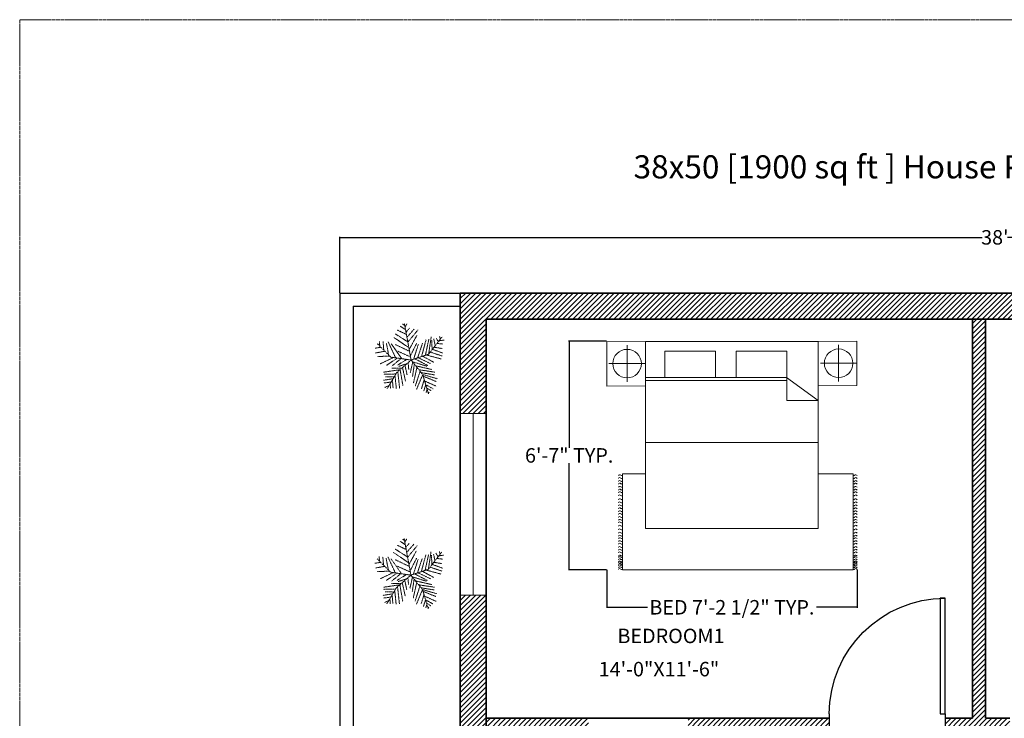
# Model space of a CAD drawing. Units: inches. Extents: x 2202345 to 2203065, y -970921 to -970107.
# Tile 4 of 5: x 2202345 to 2202685, y -970348 to -970107. Entities that reach past the tile are written whole.
import ezdxf

# ---------------------------------------------------------------- set-up
doc = ezdxf.new("R2010")
doc.units = ezdxf.units.IN
doc.header["$MEASUREMENT"] = 0
doc.linetypes.add('HIDDEN', pattern=[0.375, 0.25, -0.125])
doc.layers.get('0').update_dxf_attribs({"color": 13})
for name, color, linetype, lineweight in [('A-ANNO-DIMS', 2, 'Continuous', 18), ('A-ANNO-TEXT', 7, 'Continuous', 25), ('A-ANNO-TTLB', 7, 'HIDDEN', 18), ('A-AREA-IDEN', 7, 'Continuous', 18), ('A-WALL-PATT', 8, 'Continuous', 13), ('C-PROP', 7, 'Continuous', 25), ('doors', 252, 'Continuous', 25), ('furniture', 250, 'Continuous', 18), ('garden', 114, 'HIDDEN', 13), ('walls', 252, 'Continuous', 35), ('windows', 173, 'Continuous', 18)]:
    doc.layers.add(name, color=color, linetype=linetype, lineweight=lineweight)
doc.styles.get("Standard").update_dxf_attribs({"font": 'arial.ttf'})
doc.dimstyles.get("Standard").update_dxf_attribs({"dimtxt": 5, "dimasz": 0.18, "dimexe": 0.18, "dimexo": 0.0625, "dimgap": 0.09, "dimtad": 0, "dimtih": 1, "dimtoh": 1, "dimzin": 0, "dimdsep": 46, "dimlunit": 3, "dimtxsty": 'Standard', "dimcen": 0.09, "dimadec": 0, "dimazin": 0, "dimtfac": 1, "dimtofl": 0, "dimtmove": 0, "dimatfit": 3, "dimfxl": 1, "dimtolj": 1, "dimtzin": 0, "dimarcsym": 0})

# ---------------------------------------------------------------- blocks, each defined once
blk = doc.blocks.new('CARPET')
at = {"layer": 'furniture'}
for p, q in [((-51.53, -98.11), (-51.53, -55.12)), ((-51.53, -55.12), (-41.27, -55.12)), ((36, -55.12), (51.55, -55.12)), ((51.55, -55.12), (51.55, -98.11)), ((51.55, -98.11), (-51.53, -98.11))]:
    blk.add_line(p, q, dxfattribs=at)
for points, knots in [([(-53.37, -55.99), (-53.22, -55.8), (-52.9, -55.41), (-52.34, -55.8), (-51.89, -56.08), (-51.65, -55.91), (-51.53, -55.83)], [0, 0, 0, 0, 0.653278, 1.290138, 1.740457, 2.114451, 2.114451, 2.114451, 2.114451]), ([(-53.37, -57.26), (-53.22, -57.07), (-52.9, -56.67), (-52.34, -57.07), (-51.89, -57.35), (-51.65, -57.17), (-51.53, -57.1)], [0, 0, 0, 0, 0.653278, 1.290138, 1.740457, 2.114451, 2.114451, 2.114451, 2.114451]), ([(53.37, -55.99), (53.22, -55.8), (52.9, -55.41), (52.34, -55.8), (51.89, -56.08), (51.65, -55.91), (51.53, -55.83)], [0, 0, 0, 0, 0.653278, 1.290138, 1.740457, 2.114451, 2.114451, 2.114451, 2.114451]), ([(53.37, -57.26), (53.22, -57.07), (52.9, -56.67), (52.34, -57.07), (51.89, -57.35), (51.65, -57.17), (51.53, -57.1)], [0, 0, 0, 0, 0.653278, 1.290138, 1.740457, 2.114451, 2.114451, 2.114451, 2.114451]), ([(-53.37, -58.59), (-53.22, -58.4), (-52.9, -58.01), (-52.34, -58.4), (-51.89, -58.68), (-51.65, -58.5), (-51.53, -58.43)], [0, 0, 0, 0, 0.653278, 1.290138, 1.740457, 2.114451, 2.114451, 2.114451, 2.114451]), ([(-53.37, -59.78), (-53.22, -59.58), (-52.9, -59.19), (-52.34, -59.58), (-51.89, -59.86), (-51.65, -59.69), (-51.53, -59.61)], [0, 0, 0, 0, 0.653278, 1.290138, 1.740457, 2.114451, 2.114451, 2.114451, 2.114451]), ([(-53.37, -61.22), (-53.22, -61.02), (-52.9, -60.63), (-52.34, -61.02), (-51.89, -61.3), (-51.65, -61.13), (-51.53, -61.05)], [0, 0, 0, 0, 0.653278, 1.290138, 1.740457, 2.114451, 2.114451, 2.114451, 2.114451]), ([(53.37, -58.59), (53.22, -58.4), (52.9, -58.01), (52.34, -58.4), (51.89, -58.68), (51.65, -58.5), (51.53, -58.43)], [0, 0, 0, 0, 0.653278, 1.290138, 1.740457, 2.114451, 2.114451, 2.114451, 2.114451]), ([(53.37, -59.78), (53.22, -59.58), (52.9, -59.19), (52.34, -59.58), (51.89, -59.86), (51.65, -59.69), (51.53, -59.61)], [0, 0, 0, 0, 0.653278, 1.290138, 1.740457, 2.114451, 2.114451, 2.114451, 2.114451]), ([(53.37, -61.22), (53.22, -61.02), (52.9, -60.63), (52.34, -61.02), (51.89, -61.3), (51.65, -61.13), (51.53, -61.05)], [0, 0, 0, 0, 0.653278, 1.290138, 1.740457, 2.114451, 2.114451, 2.114451, 2.114451]), ([(-53.37, -62.44), (-53.22, -62.25), (-52.9, -61.86), (-52.34, -62.25), (-51.89, -62.53), (-51.65, -62.36), (-51.53, -62.28)], [0, 0, 0, 0, 0.653278, 1.290138, 1.740457, 2.114451, 2.114451, 2.114451, 2.114451]), ([(-53.37, -63.63), (-53.22, -63.43), (-52.9, -63.04), (-52.34, -63.43), (-51.89, -63.72), (-51.65, -63.54), (-51.53, -63.46)], [0, 0, 0, 0, 0.653278, 1.290138, 1.740457, 2.114451, 2.114451, 2.114451, 2.114451]), ([(-53.37, -65.07), (-53.22, -64.87), (-52.9, -64.48), (-52.34, -64.87), (-51.89, -65.15), (-51.65, -64.98), (-51.53, -64.9)], [0, 0, 0, 0, 0.653278, 1.290138, 1.740457, 2.114451, 2.114451, 2.114451, 2.114451]), ([(53.37, -62.44), (53.22, -62.25), (52.9, -61.86), (52.34, -62.25), (51.89, -62.53), (51.65, -62.36), (51.53, -62.28)], [0, 0, 0, 0, 0.653278, 1.290138, 1.740457, 2.114451, 2.114451, 2.114451, 2.114451]), ([(53.37, -63.63), (53.22, -63.43), (52.9, -63.04), (52.34, -63.43), (51.89, -63.72), (51.65, -63.54), (51.53, -63.46)], [0, 0, 0, 0, 0.653278, 1.290138, 1.740457, 2.114451, 2.114451, 2.114451, 2.114451]), ([(53.37, -65.07), (53.22, -64.87), (52.9, -64.48), (52.34, -64.87), (51.89, -65.15), (51.65, -64.98), (51.53, -64.9)], [0, 0, 0, 0, 0.653278, 1.290138, 1.740457, 2.114451, 2.114451, 2.114451, 2.114451]), ([(-53.37, -66.76), (-53.22, -66.56), (-52.9, -66.17), (-52.34, -66.56), (-51.89, -66.84), (-51.65, -66.67), (-51.53, -66.59)], [0, 0, 0, 0, 0.653278, 1.290138, 1.740457, 2.114451, 2.114451, 2.114451, 2.114451]), ([(-53.37, -68.2), (-53.22, -68), (-52.9, -67.61), (-52.34, -68), (-51.89, -68.28), (-51.65, -68.11), (-51.53, -68.03)], [0, 0, 0, 0, 0.653278, 1.290138, 1.740457, 2.114451, 2.114451, 2.114451, 2.114451]), ([(-53.37, -69.53), (-53.22, -69.33), (-52.9, -68.94), (-52.34, -69.33), (-51.89, -69.61), (-51.65, -69.44), (-51.53, -69.36)], [0, 0, 0, 0, 0.653278, 1.290138, 1.740457, 2.114451, 2.114451, 2.114451, 2.114451]), ([(-53.37, -70.79), (-53.22, -70.6), (-52.9, -70.21), (-52.34, -70.6), (-51.89, -70.88), (-51.65, -70.7), (-51.53, -70.63)], [0, 0, 0, 0, 0.653278, 1.290138, 1.740457, 2.114451, 2.114451, 2.114451, 2.114451]), ([(53.37, -66.76), (53.22, -66.56), (52.9, -66.17), (52.34, -66.56), (51.89, -66.84), (51.65, -66.67), (51.53, -66.59)], [0, 0, 0, 0, 0.653278, 1.290138, 1.740457, 2.114451, 2.114451, 2.114451, 2.114451]), ([(53.37, -68.2), (53.22, -68), (52.9, -67.61), (52.34, -68), (51.89, -68.28), (51.65, -68.11), (51.53, -68.03)], [0, 0, 0, 0, 0.653278, 1.290138, 1.740457, 2.114451, 2.114451, 2.114451, 2.114451]), ([(53.37, -69.53), (53.22, -69.33), (52.9, -68.94), (52.34, -69.33), (51.89, -69.61), (51.65, -69.44), (51.53, -69.36)], [0, 0, 0, 0, 0.653278, 1.290138, 1.740457, 2.114451, 2.114451, 2.114451, 2.114451]), ([(53.37, -70.79), (53.22, -70.6), (52.9, -70.21), (52.34, -70.6), (51.89, -70.88), (51.65, -70.7), (51.53, -70.63)], [0, 0, 0, 0, 0.653278, 1.290138, 1.740457, 2.114451, 2.114451, 2.114451, 2.114451]), ([(-53.37, -72.12), (-53.22, -71.93), (-52.9, -71.54), (-52.34, -71.93), (-51.89, -72.21), (-51.65, -72.04), (-51.53, -71.96)], [0, 0, 0, 0, 0.653278, 1.290138, 1.740457, 2.114451, 2.114451, 2.114451, 2.114451]), ([(-53.37, -73.31), (-53.22, -73.11), (-52.9, -72.72), (-52.34, -73.11), (-51.89, -73.4), (-51.65, -73.22), (-51.53, -73.14)], [0, 0, 0, 0, 0.653278, 1.290138, 1.740457, 2.114451, 2.114451, 2.114451, 2.114451]), ([(-53.37, -74.75), (-53.22, -74.55), (-52.9, -74.16), (-52.34, -74.55), (-51.89, -74.83), (-51.65, -74.66), (-51.53, -74.58)], [0, 0, 0, 0, 0.653278, 1.290138, 1.740457, 2.114451, 2.114451, 2.114451, 2.114451]), ([(53.37, -72.12), (53.22, -71.93), (52.9, -71.54), (52.34, -71.93), (51.89, -72.21), (51.65, -72.04), (51.53, -71.96)], [0, 0, 0, 0, 0.653278, 1.290138, 1.740457, 2.114451, 2.114451, 2.114451, 2.114451]), ([(53.37, -73.31), (53.22, -73.11), (52.9, -72.72), (52.34, -73.11), (51.89, -73.4), (51.65, -73.22), (51.53, -73.14)], [0, 0, 0, 0, 0.653278, 1.290138, 1.740457, 2.114451, 2.114451, 2.114451, 2.114451]), ([(53.37, -74.75), (53.22, -74.55), (52.9, -74.16), (52.34, -74.55), (51.89, -74.83), (51.65, -74.66), (51.53, -74.58)], [0, 0, 0, 0, 0.653278, 1.290138, 1.740457, 2.114451, 2.114451, 2.114451, 2.114451]), ([(-53.37, -75.98), (-53.22, -75.78), (-52.9, -75.39), (-52.34, -75.78), (-51.89, -76.06), (-51.65, -75.89), (-51.53, -75.81)], [0, 0, 0, 0, 0.653278, 1.290138, 1.740457, 2.114451, 2.114451, 2.114451, 2.114451]), ([(-53.37, -77.16), (-53.22, -76.96), (-52.9, -76.57), (-52.34, -76.96), (-51.89, -77.25), (-51.65, -77.07), (-51.53, -76.99)], [0, 0, 0, 0, 0.653278, 1.290138, 1.740457, 2.114451, 2.114451, 2.114451, 2.114451]), ([(-53.37, -78.6), (-53.22, -78.4), (-52.9, -78.01), (-52.34, -78.4), (-51.89, -78.68), (-51.65, -78.51), (-51.53, -78.43)], [0, 0, 0, 0, 0.653278, 1.290138, 1.740457, 2.114451, 2.114451, 2.114451, 2.114451]), ([(53.37, -75.98), (53.22, -75.78), (52.9, -75.39), (52.34, -75.78), (51.89, -76.06), (51.65, -75.89), (51.53, -75.81)], [0, 0, 0, 0, 0.653278, 1.290138, 1.740457, 2.114451, 2.114451, 2.114451, 2.114451]), ([(53.37, -77.16), (53.22, -76.96), (52.9, -76.57), (52.34, -76.96), (51.89, -77.25), (51.65, -77.07), (51.53, -76.99)], [0, 0, 0, 0, 0.653278, 1.290138, 1.740457, 2.114451, 2.114451, 2.114451, 2.114451]), ([(53.37, -78.6), (53.22, -78.4), (52.9, -78.01), (52.34, -78.4), (51.89, -78.68), (51.65, -78.51), (51.53, -78.43)], [0, 0, 0, 0, 0.653278, 1.290138, 1.740457, 2.114451, 2.114451, 2.114451, 2.114451]), ([(-53.37, -80.29), (-53.22, -80.09), (-52.9, -79.7), (-52.34, -80.09), (-51.89, -80.37), (-51.65, -80.2), (-51.53, -80.12)], [0, 0, 0, 0, 0.653278, 1.290138, 1.740457, 2.114451, 2.114451, 2.114451, 2.114451]), ([(-53.37, -81.73), (-53.22, -81.53), (-52.9, -81.14), (-52.34, -81.53), (-51.89, -81.81), (-51.65, -81.64), (-51.53, -81.56)], [0, 0, 0, 0, 0.653278, 1.290138, 1.740457, 2.114451, 2.114451, 2.114451, 2.114451]), ([(-53.37, -83.06), (-53.22, -82.86), (-52.9, -82.47), (-52.34, -82.86), (-51.89, -83.14), (-51.65, -82.97), (-51.53, -82.89)], [0, 0, 0, 0, 0.653278, 1.290138, 1.740457, 2.114451, 2.114451, 2.114451, 2.114451]), ([(53.37, -80.29), (53.22, -80.09), (52.9, -79.7), (52.34, -80.09), (51.89, -80.37), (51.65, -80.2), (51.53, -80.12)], [0, 0, 0, 0, 0.653278, 1.290138, 1.740457, 2.114451, 2.114451, 2.114451, 2.114451]), ([(53.37, -81.73), (53.22, -81.53), (52.9, -81.14), (52.34, -81.53), (51.89, -81.81), (51.65, -81.64), (51.53, -81.56)], [0, 0, 0, 0, 0.653278, 1.290138, 1.740457, 2.114451, 2.114451, 2.114451, 2.114451]), ([(53.37, -83.06), (53.22, -82.86), (52.9, -82.47), (52.34, -82.86), (51.89, -83.14), (51.65, -82.97), (51.53, -82.89)], [0, 0, 0, 0, 0.653278, 1.290138, 1.740457, 2.114451, 2.114451, 2.114451, 2.114451]), ([(-53.37, -84.18), (-53.22, -83.99), (-52.9, -83.6), (-52.34, -83.99), (-51.89, -84.27), (-51.65, -84.09), (-51.53, -84.02)], [0, 0, 0, 0, 0.653278, 1.290138, 1.740457, 2.114451, 2.114451, 2.114451, 2.114451]), ([(-53.37, -85.51), (-53.22, -85.32), (-52.9, -84.93), (-52.34, -85.32), (-51.89, -85.6), (-51.65, -85.42), (-51.53, -85.35)], [0, 0, 0, 0, 0.653278, 1.290138, 1.740457, 2.114451, 2.114451, 2.114451, 2.114451]), ([(-53.37, -86.7), (-53.22, -86.5), (-52.9, -86.11), (-52.34, -86.5), (-51.89, -86.78), (-51.65, -86.61), (-51.53, -86.53)], [0, 0, 0, 0, 0.653278, 1.290138, 1.740457, 2.114451, 2.114451, 2.114451, 2.114451]), ([(-53.37, -88.14), (-53.22, -87.94), (-52.9, -87.55), (-52.34, -87.94), (-51.89, -88.22), (-51.65, -88.05), (-51.53, -87.97)], [0, 0, 0, 0, 0.653278, 1.290138, 1.740457, 2.114451, 2.114451, 2.114451, 2.114451]), ([(53.37, -84.18), (53.22, -83.99), (52.9, -83.6), (52.34, -83.99), (51.89, -84.27), (51.65, -84.09), (51.53, -84.02)], [0, 0, 0, 0, 0.653278, 1.290138, 1.740457, 2.114451, 2.114451, 2.114451, 2.114451]), ([(53.37, -85.51), (53.22, -85.32), (52.9, -84.93), (52.34, -85.32), (51.89, -85.6), (51.65, -85.42), (51.53, -85.35)], [0, 0, 0, 0, 0.653278, 1.290138, 1.740457, 2.114451, 2.114451, 2.114451, 2.114451]), ([(53.37, -86.7), (53.22, -86.5), (52.9, -86.11), (52.34, -86.5), (51.89, -86.78), (51.65, -86.61), (51.53, -86.53)], [0, 0, 0, 0, 0.653278, 1.290138, 1.740457, 2.114451, 2.114451, 2.114451, 2.114451]), ([(53.37, -88.14), (53.22, -87.94), (52.9, -87.55), (52.34, -87.94), (51.89, -88.22), (51.65, -88.05), (51.53, -87.97)], [0, 0, 0, 0, 0.653278, 1.290138, 1.740457, 2.114451, 2.114451, 2.114451, 2.114451]), ([(-53.37, -89.36), (-53.22, -89.17), (-52.9, -88.78), (-52.34, -89.17), (-51.89, -89.45), (-51.65, -89.28), (-51.53, -89.2)], [0, 0, 0, 0, 0.653278, 1.290138, 1.740457, 2.114451, 2.114451, 2.114451, 2.114451]), ([(-53.37, -90.55), (-53.22, -90.35), (-52.9, -89.96), (-52.34, -90.35), (-51.89, -90.64), (-51.65, -90.46), (-51.53, -90.38)], [0, 0, 0, 0, 0.653278, 1.290138, 1.740457, 2.114451, 2.114451, 2.114451, 2.114451]), ([(-53.37, -91.99), (-53.22, -91.79), (-52.9, -91.4), (-52.34, -91.79), (-51.89, -92.07), (-51.65, -91.9), (-51.53, -91.82)], [0, 0, 0, 0, 0.653278, 1.290138, 1.740457, 2.114451, 2.114451, 2.114451, 2.114451]), ([(-53.37, -92.69), (-53.22, -92.48), (-52.9, -92.08), (-52.35, -92.49), (-51.89, -92.77), (-51.65, -92.6), (-51.53, -92.52)], [0, 0, 0, 0, 0.663904, 1.307406, 1.757725, 2.131719, 2.131719, 2.131719, 2.131719]), ([(53.37, -89.36), (53.22, -89.17), (52.9, -88.78), (52.34, -89.17), (51.89, -89.45), (51.65, -89.28), (51.53, -89.2)], [0, 0, 0, 0, 0.653278, 1.290138, 1.740457, 2.114451, 2.114451, 2.114451, 2.114451]), ([(53.37, -90.55), (53.22, -90.35), (52.9, -89.96), (52.34, -90.35), (51.9, -90.63), (51.66, -90.47), (51.55, -90.4)], [0, 0, 0, 0, 0.653278, 1.290138, 1.740457, 2.0926, 2.0926, 2.0926, 2.0926]), ([(53.37, -91.99), (53.22, -91.79), (52.9, -91.4), (52.34, -91.79), (51.9, -92.07), (51.66, -91.91), (51.55, -91.83)], [0, 0, 0, 0, 0.653278, 1.290138, 1.740457, 2.0926, 2.0926, 2.0926, 2.0926]), ([(53.37, -92.69), (53.22, -92.49), (52.9, -92.09), (52.34, -92.49), (51.9, -92.77), (51.66, -92.61), (51.55, -92.53)], [0, 0, 0, 0, 0.656792, 1.295826, 1.746145, 2.098292, 2.098292, 2.098292, 2.098292]), ([(-53.37, -93.61), (-53.22, -93.42), (-52.9, -93.03), (-52.34, -93.42), (-51.89, -93.7), (-51.65, -93.52), (-51.53, -93.45)], [0, 0, 0, 0, 0.653278, 1.290138, 1.740457, 2.114451, 2.114451, 2.114451, 2.114451]), ([(-53.37, -94.55), (-53.22, -94.35), (-52.9, -93.96), (-52.34, -94.35), (-51.89, -94.63), (-51.65, -94.46), (-51.53, -94.38)], [0, 0, 0, 0, 0.653278, 1.290138, 1.740457, 2.114451, 2.114451, 2.114451, 2.114451]), ([(-53.37, -95.05), (-53.22, -94.85), (-52.9, -94.46), (-52.34, -94.85), (-51.89, -95.14), (-51.65, -94.96), (-51.53, -94.88)], [0, 0, 0, 0, 0.653278, 1.290138, 1.740457, 2.114451, 2.114451, 2.114451, 2.114451]), ([(-53.37, -95.73), (-53.22, -95.54), (-52.9, -95.15), (-52.34, -95.54), (-51.89, -95.82), (-51.65, -95.65), (-51.53, -95.57)], [0, 0, 0, 0, 0.653278, 1.290138, 1.740457, 2.114451, 2.114451, 2.114451, 2.114451]), ([(-53.37, -96.38), (-53.22, -96.18), (-52.9, -95.79), (-52.34, -96.18), (-51.89, -96.47), (-51.65, -96.29), (-51.53, -96.21)], [0, 0, 0, 0, 0.653278, 1.290138, 1.740457, 2.114451, 2.114451, 2.114451, 2.114451]), ([(-53.37, -97.17), (-53.22, -96.98), (-52.9, -96.59), (-52.34, -96.98), (-51.89, -97.26), (-51.65, -97.08), (-51.53, -97.01)], [0, 0, 0, 0, 0.653278, 1.290138, 1.740457, 2.114451, 2.114451, 2.114451, 2.114451]), ([(53.37, -95.78), (53.22, -95.58), (52.9, -95.19), (52.34, -95.58), (51.89, -95.86), (51.65, -95.69), (51.53, -95.61)], [0, 0, 0, 0, 0.653278, 1.290138, 1.740457, 2.114451, 2.114451, 2.114451, 2.114451]), ([(53.37, -96.43), (53.22, -96.23), (52.9, -95.84), (52.34, -96.23), (51.89, -96.51), (51.65, -96.34), (51.53, -96.26)], [0, 0, 0, 0, 0.653278, 1.290138, 1.740457, 2.114451, 2.114451, 2.114451, 2.114451]), ([(53.37, -97.22), (53.22, -97.02), (52.9, -96.63), (52.34, -97.02), (51.89, -97.3), (51.65, -97.13), (51.53, -97.05)], [0, 0, 0, 0, 0.653278, 1.290138, 1.740457, 2.114451, 2.114451, 2.114451, 2.114451]), ([(53.37, -93.66), (53.22, -93.46), (52.9, -93.07), (52.34, -93.46), (51.9, -93.74), (51.66, -93.58), (51.55, -93.5)], [0, 0, 0, 0, 0.653278, 1.290138, 1.740457, 2.0926, 2.0926, 2.0926, 2.0926]), ([(53.37, -94.59), (53.22, -94.4), (52.9, -94.01), (52.34, -94.4), (51.9, -94.68), (51.66, -94.51), (51.55, -94.44)], [0, 0, 0, 0, 0.653278, 1.290138, 1.740457, 2.0926, 2.0926, 2.0926, 2.0926]), ([(53.37, -95.1), (53.22, -94.9), (52.9, -94.51), (52.34, -94.9), (51.9, -95.18), (51.66, -95.02), (51.55, -94.94)], [0, 0, 0, 0, 0.653278, 1.290138, 1.740457, 2.0926, 2.0926, 2.0926, 2.0926]), ([(-53.37, -97.99), (-53.22, -97.79), (-52.9, -97.4), (-52.34, -97.79), (-51.89, -98.08), (-51.65, -97.9), (-51.53, -97.82)], [0, 0, 0, 0, 0.653278, 1.290138, 1.740457, 2.114451, 2.114451, 2.114451, 2.114451]), ([(53.37, -97.99), (53.22, -97.79), (52.9, -97.4), (52.34, -97.79), (51.89, -98.08), (51.65, -97.9), (51.53, -97.82)], [0, 0, 0, 0, 0.653278, 1.290138, 1.740457, 2.114451, 2.114451, 2.114451, 2.114451])]:
    blk.add_open_spline(points, degree=3, knots=knots, dxfattribs=at)
blk = doc.blocks.new('A$C58D270C6')
at = {"layer": 'furniture'}
for p, q in [((9.09, 124.13), (9.09, 108.87)), ((1.46, 116.5), (16.73, 116.5)), ((14.97, 94.84), (24.62, 107.92)), ((24.62, 94.93), (24.62, 107.92)), ((42.08, 108), (42.08, 36)), ((14.97, 94.93), (24.62, 94.93)), ((14.97, 94.84), (14.97, 36)), ((16.22, 94.93), (16.22, 36)), ((9.25, 36), (9.25, 20.74)), ((1.62, 28.37), (16.88, 28.37))]:
    blk.add_line(p, q, dxfattribs=at)
for points in [[(18.5, 108), (18.34, 124.13), (-0.16, 124.13), (0, 108)], [(0, 108), (77.91, 108), (77.91, 36), (0, 36)], [(4.09, 94.93), (14.97, 94.93), (14.97, 73.83), (4.09, 73.83)], [(4.09, 65.23), (14.97, 65.23), (14.97, 44.13), (4.09, 44.13)], [(18.65, 19.87), (18.5, 36), (0, 36), (0.16, 19.87)]]:
    blk.add_lwpolyline(points, close=True, dxfattribs=at)
for centre in [(9.09, 116.5), (9.25, 28.37)]:
    blk.add_circle(centre, 5.95, dxfattribs=at)
at = {"layer": 'furniture', "xscale": 0.9312884925094044, "yscale": 0.9312884925094044, "zscale": 0.9312884925094044, "rotation": 90}
blk.add_blockref('CARPET', (3.79, 74.47), dxfattribs=at)
blk = doc.blocks.new('*U12')
for p, q in [((0, 0), (0, -6)), ((40, 0), (40, -6))]:
    blk.add_line(p, q)
blk.add_lwpolyline([(0, 0), (0, 40), (1.75, 40), (1.75, 0)], close=True)
blk.add_arc((0, 0), 40, 0, 90)
blk = doc.blocks.new('*D20')
at = {"layer": 'A-ANNO-DIMS', "color": 0, "lineweight": -2, "transparency": 16777216}
for p, q in [((2202455.18, -970201.04), (2202455.18, -970181.68)), ((2202455.36, -970181.86), (2202677.1, -970181.86)), ((2202907.5, -970181.86), (2202685.76, -970181.86)), ((2202907.68, -970201.04), (2202907.68, -970181.68))]:
    blk.add_line(p, q, dxfattribs=at)
at = {"layer": 'A-ANNO-DIMS', "color": 0, "transparency": 16777216}
for points in [[(2202455.36, -970181.83), (2202455.36, -970181.89), (2202455.18, -970181.86)], [(2202907.5, -970181.83), (2202907.5, -970181.89), (2202907.68, -970181.86)]]:
    blk.add_solid(points, dxfattribs=at)
at = {"layer": 'Defpoints', "color": 0, "transparency": 16777216}
for p in [(2202907.68, -970181.86), (2202455.18, -970201.11), (2202907.68, -970201.11)]:
    blk.add_point(p, dxfattribs=at)
at = {"layer": 'A-ANNO-DIMS', "color": 0, "transparency": 16777216, "insert": (2202681.43, -970181.86), "char_height": 5, "attachment_point": 5}
blk.add_mtext("\\A1;38'", dxfattribs=at)
blk = doc.blocks.new('*U23')
for p, q in [((-7.288, 39.707), (-21.778, 46.673)), ((-8.737, 47.138), (-17.069, 52.711)), ((-10.186, 53.64), (-13.084, 55.962)), ((0, 0), (-10.5, 57)), ((-9.099, 51.782), (-6.563, 55.962)), ((-7.65, 43.423), (-2.578, 49.46)), ((-5.839, 35.992), (4.667, 48.067)), ((-5.114, 27.632), (10.463, 46.673)), ((-3.665, 19.273), (-27.574, 35.527)), ((-5.114, 28.097), (-24.676, 40.636)), ((-2.941, 16.486), (8.652, 37.85)), ((16.259, 5.805), (23.142, 31.348)), ((22.055, 7.198), (27.489, 32.277)), ((27, 9), (48, 36)), ((27.127, 9.056), (31.112, 35.992)), ((31.836, 30.883), (32.561, 16.486)), ((35.096, 32.741), (37.27, 22.524)), ((38.719, 34.134), (41.979, 28.561)), ((43.791, 29.954), (51.036, 30.883)), ((44.153, 36.456), (45.239, 32.741)), ((-47.498, 19.737), (-55.83, 18.344)), ((-31.5, 4.5), (-52.5, 25.5)), ((-48.585, 21.131), (-49.309, 29.026)), ((-43.513, 28.561), (-42.427, 15.558)), ((-38.442, 26.239), (-34.819, 7.663)), ((-35.544, 28.097), (-24.314, 3.947)), ((-14.533, 2.09), (-30.834, 25.31)), ((-24.314, 23.917), (-2.941, 13.7)), ((-1.129, 6.734), (9.014, 26.704)), ((3.942, 1.625), (11.187, 24.381)), ((10.101, 3.483), (17.708, 26.239)), ((33.285, 16.486), (48.862, 10.913)), ((36.183, 19.737), (48.137, 17.88)), ((40.53, 25.775), (48.862, 24.846)), ((-40.615, 13.7), (-55.105, 10.913)), ((-33.37, 6.269), (-52.207, 5.34)), ((-28.299, 3.483), (-47.86, -5.805)), ((-21.416, 3.018), (-38.079, -8.128)), ((0, 0), (-31.5, 4.5)), ((-15.982, 2.09), (-30.11, -9.521)), ((0, 0), (-22.5, -19.5)), ((-6.563, 1.161), (-21.416, -8.128)), ((-20.691, 13.7), (-1.129, 4.876)), ((0, 0), (27, 9)), ((0, 0), (18, -22.5)), ((6.478, 1.625), (26.04, -8.592)), ((11.187, 3.483), (30.749, -5.805)), ((18.07, 5.805), (35.096, -3.483)), ((24.229, 7.663), (46.688, 1.625)), ((29.662, 12.307), (48.137, 6.269)), ((-17.431, -15.094), (-42.789, -18.809)), ((-15.257, -12.772), (-30.11, -12.772)), ((-6.563, -5.805), (-19.967, -9.985)), ((-17.069, -15.094), (-12.721, -40.172)), ((-13.446, -11.378), (-8.737, -32.741)), ((-9.461, -8.592), (-6.201, -23.453)), ((-4.752, -3.483), (-3.665, -14.629)), ((2.493, -3.019), (-1.491, -20.202)), ((1.769, -2.555), (24.229, -9.521)), ((5.029, -6.27), (2.131, -25.775)), ((9.014, -11.378), (3.58, -35.992)), ((7.565, -9.056), (32.198, -14.629)), ((12.274, -15.094), (36.907, -18.809)), ((-28.299, -29.026), (-42.789, -31.348)), ((-24.314, -21.596), (-42.427, -22.06)), ((-26.849, -26.24), (-40.253, -25.775)), ((-22.5, -19.5), (-37.5, -45)), ((-25.038, -23.918), (-22.865, -45.281)), ((-20.691, -18.345), (-17.793, -44.352)), ((14.085, -16.951), (6.478, -40.172)), ((18.07, -22.524), (8.289, -45.745)), ((20.244, -30.419), (15.897, -44.816)), ((16.259, -19.738), (36.183, -22.989)), ((18, -22.5), (27, -52.5)), ((18.433, -22.524), (40.53, -29.026)), ((19.157, -25.311), (38.719, -33.206)), ((-30.834, -34.135), (-42.427, -35.528)), ((-34.457, -39.708), (-40.978, -42.494)), ((-32.646, -36.921), (-31.921, -44.352)), ((-29.023, -30.884), (-27.936, -43.887)), ((22.78, -37.85), (19.519, -48.532)), ((21.331, -32.741), (39.081, -40.636)), ((22.78, -38.314), (34.372, -44.816)), ((24.591, -45.745), (23.142, -50.854)), ((24.591, -43.423), (30.749, -47.603)), ((26.764, -49.925), (28.213, -50.854))]:
    blk.add_line(p, q)
blk = doc.blocks.new('*D25')
at = {"layer": 'A-ANNO-DIMS', "color": 0, "lineweight": -2, "transparency": 16777216}
for p, q in [((2202547.33, -970296.82), (2202547.33, -970309.91)), ((2202633.84, -970296.82), (2202633.84, -970309.91)), ((2202547.51, -970309.73), (2202561.39, -970309.73)), ((2202633.66, -970309.73), (2202619.78, -970309.73))]:
    blk.add_line(p, q, dxfattribs=at)
at = {"layer": 'A-ANNO-DIMS', "color": 0, "transparency": 16777216}
for points in [[(2202547.51, -970309.7), (2202547.51, -970309.76), (2202547.33, -970309.73)], [(2202633.66, -970309.7), (2202633.66, -970309.76), (2202633.84, -970309.73)]]:
    blk.add_solid(points, dxfattribs=at)
at = {"layer": 'Defpoints', "color": 0, "transparency": 16777216}
for p in [(2202547.33, -970296.75), (2202633.84, -970296.75), (2202633.84, -970309.73)]:
    blk.add_point(p, dxfattribs=at)
at = {"layer": 'A-ANNO-DIMS', "color": 0, "transparency": 16777216, "insert": (2202590.58, -970309.73), "char_height": 5, "attachment_point": 5}
blk.add_mtext('\\A1;BED 7\'-2 1/2" TYP.', dxfattribs=at)
blk = doc.blocks.new('*D26')
at = {"layer": 'A-ANNO-DIMS', "color": 0, "lineweight": -2, "transparency": 16777216}
for p, q in [((2202547.27, -970217.71), (2202534.18, -970217.71)), ((2202534.36, -970217.89), (2202534.36, -970254.59)), ((2202534.36, -970296.57), (2202534.36, -970259.88)), ((2202547.27, -970296.75), (2202534.18, -970296.75))]:
    blk.add_line(p, q, dxfattribs=at)
at = {"layer": 'A-ANNO-DIMS', "color": 0, "transparency": 16777216}
for points in [[(2202534.33, -970217.89), (2202534.39, -970217.89), (2202534.36, -970217.71)], [(2202534.33, -970296.57), (2202534.39, -970296.57), (2202534.36, -970296.75)]]:
    blk.add_solid(points, dxfattribs=at)
at = {"layer": 'Defpoints', "color": 0, "transparency": 16777216}
for p in [(2202547.33, -970217.71), (2202534.36, -970296.75), (2202547.33, -970296.75)]:
    blk.add_point(p, dxfattribs=at)
at = {"layer": 'A-ANNO-DIMS', "color": 0, "transparency": 16777216, "insert": (2202534.36, -970257.23), "char_height": 5, "attachment_point": 5}
blk.add_mtext('\\A1;6\'-7" TYP.', dxfattribs=at)

msp = doc.modelspace()

# ---------------------------------------------------------------- hatches: boundary and pattern name
at = {"layer": 'A-WALL-PATT'}
h = msp.add_hatch(dxfattribs=at)
h.set_pattern_fill('ANSI31', color=256, scale=10)
h.set_pattern_definition([(45, (0, 0), (-0.8838834765, 0.8838834765), [])])
h.paths.add_polyline_path([(2202648.182, -970512.768), (2202644.707, -970512.768, -0.0110733), (2202643.682, -970512.746), (2202643.682, -970601.606), (2202609.913, -970601.606), (2202609.913, -970610.606), (2202643.682, -970610.606), (2202643.682, -970619.168), (2202647.677, -970619.168, -0.0047326), (2202648.182, -970619.173)])
h.paths.add_polyline_path([(2202643.682, -970610.606), (2202636.037, -970610.606), (2202636.037, -970659.106), (2202643.682, -970659.106)])
h.paths.add_polyline_path([(2202722.39, -970654.606), (2202722.39, -970650.106), (2202648.182, -970650.106), (2202648.182, -970645.806), (2202647.677, -970645.806), (2202643.682, -970645.806), (2202643.682, -970659.106), (2202722.39, -970659.106)])
h.paths.add_polyline_path([(2202846.182, -970650.106), (2202798.148, -970650.106), (2202798.148, -970659.106), (2202846.182, -970659.106)])
h.paths.add_polyline_path([(2202855.182, -970619.995), (2202846.182, -970619.995), (2202846.182, -970682.124), (2202855.182, -970682.124)])
h.paths.add_polyline_path([(2202855.182, -970434.646), (2202846.182, -970434.646), (2202846.182, -970545.038), (2202855.182, -970545.038)])
h.paths.add_polyline_path([(2202903.182, -970745.106), (2202855.182, -970745.106), (2202855.182, -970729.208), (2202846.182, -970729.208), (2202846.182, -970745.106), (2202725.91, -970745.106), (2202725.91, -970754.106), (2202903.182, -970754.106)])
h.paths.add_polyline_path([(2202846.182, -970489.606), (2202767.486, -970489.606, -0.1570508), (2202766.685, -970489.864), (2202739.229, -970489.864, -0.1570508), (2202738.428, -970489.606), (2202685.343, -970489.606), (2202685.343, -970494.106), (2202846.182, -970494.106)])
h.paths.add_polyline_path([(2202648.182, -970477.106), (2202594.182, -970477.106), (2202594.182, -970352.606), (2202624.243, -970352.606), (2202624.243, -970348.106), (2202575.482, -970348.106), (2202575.482, -970352.606), (2202589.682, -970352.606), (2202589.682, -970412.606), (2202505.682, -970412.606), (2202505.682, -970417.106), (2202589.682, -970417.106), (2202589.682, -970477.106), (2202580.925, -970477.106), (2202580.925, -970481.606), (2202643.682, -970481.606), (2202643.682, -970489.606), (2202644.707, -970489.606), (2202648.182, -970489.606)])
h.paths.add_polyline_path([(2202505.682, -970305.515), (2202496.682, -970305.515), (2202496.682, -970378.877), (2202501.298, -970378.877), (2202505.682, -970378.877)])
h.paths.add_polyline_path([(2202540.998, -970348.106), (2202505.682, -970348.106), (2202505.682, -970352.606), (2202540.998, -970352.606)], flags=17)
h.paths.add_polyline_path([(2202505.682, -970452.918), (2202496.682, -970452.918), (2202496.682, -970516.267), (2202505.682, -970516.267)])
h.paths.add_polyline_path([(2202505.682, -970210.106), (2202898.682, -970210.106), (2202898.682, -970294.106), (2202889.459, -970294.106), (2202889.459, -970303.106), (2202907.682, -970303.106), (2202907.682, -970201.106), (2202496.682, -970201.106), (2202496.682, -970242.728), (2202505.682, -970242.728)])
h.paths.add_polyline_path([(2202678.182, -970210.106), (2202673.682, -970210.106), (2202673.682, -970348.106), (2202664.243, -970348.106), (2202664.243, -970352.606), (2202686.569, -970352.606), (2202686.569, -970348.106), (2202678.182, -970348.106)])
h.paths.add_polyline_path([(2202752.572, -970321.843), (2202794.204, -970321.843), (2202794.204, -970314.185), (2202752.572, -970314.185)], flags=9)
h.paths.add_polyline_path([(2202750.562, -970312.127), (2202793.125, -970312.127), (2202793.125, -970304.366), (2202750.562, -970304.366)], flags=9)

# ---------------------------------------------------------------- linework, layer by layer
at = {"layer": 'A-ANNO-TTLB'}
for p, q in [((2202344.52, -970106.63), (2202344.52, -970920.555)), ((2203064.943, -970106.63), (2202344.52, -970106.63))]:
    msp.add_line(p, q, dxfattribs=at)
at = {"layer": 'C-PROP'}
for p, q in [((2202455.182, -970201.106), (2202455.182, -970804.606)), ((2202455.182, -970201.106), (2202496.682, -970201.106)), ((2202459.682, -970205.606), (2202459.682, -970800.106)), ((2202459.682, -970205.606), (2202496.682, -970205.606))]:
    msp.add_line(p, q, dxfattribs=at)
at = {"layer": 'walls'}
for p, q in [((2202496.682, -970201.106), (2202907.682, -970201.106)), ((2202496.682, -970201.106), (2202496.682, -970610.606)), ((2202505.682, -970210.106), (2202505.682, -970601.606)), ((2202505.682, -970210.106), (2202898.682, -970210.106)), ((2202673.682, -970210.106), (2202673.682, -970348.106)), ((2202678.182, -970210.106), (2202678.182, -970348.106)), ((2202505.682, -970348.106), (2202624.243, -970348.106)), ((2202664.243, -970348.106), (2202673.682, -970348.106)), ((2202678.182, -970348.106), (2202686.569, -970348.106))]:
    msp.add_line(p, q, dxfattribs=at)
at = {"layer": 'windows'}
for p, q in [((2202496.682, -970242.728), (2202505.682, -970242.728)), ((2202505.682, -970242.728), (2202501.182, -970242.728)), ((2202501.182, -970242.728), (2202501.182, -970305.515)), ((2202501.182, -970305.515), (2202496.682, -970305.515)), ((2202496.682, -970305.515), (2202505.682, -970305.515))]:
    msp.add_line(p, q, dxfattribs=at)

# ---------------------------------------------------------------- block references
at = {"layer": 'doors', "xscale": -1}
msp.add_blockref('*U12', (2202664.243, -970346.606), dxfattribs=at)
at = {"layer": 'furniture', "xscale": 0.8292897843380787, "yscale": 0.8292897843380787, "zscale": 0.8292897843380787, "rotation": 270}
msp.add_blockref('A$C58D270C6', (2202530.854, -970217.841), dxfattribs=at)
at = {"layer": 'garden', "xscale": 0.2228486455557245, "yscale": 0.2228486455557245, "zscale": 0.2228486455557245}
for p in [(2202479.762, -970224.271), (2202479.681, -970298.612)]:
    msp.add_blockref('*U23', p, dxfattribs=at)

# ---------------------------------------------------------------- texts
at = {"layer": 'A-ANNO-TEXT'}
msp.add_text('38x50 [1900 sq ft ] House Plan - West face - FP1317', height=8, dxfattribs=at).set_placement((2202556.608, -970161.49))
at = {"layer": 'A-AREA-IDEN'}
for s, p in [('BEDROOM1', (2202551.041, -970322.127)), ('14\'-0"X11\'-6"', (2202544.584, -970333.598))]:
    msp.add_text(s, height=5, dxfattribs=at).set_placement(p)

# ---------------------------------------------------------------- dimensions: what is measured, and where the dimension line sits
at = {"layer": 'A-ANNO-DIMS'}
for base, p1, p2, text, override, picture, middle in [((2202907.682, -970181.861), (2202455.182, -970201.106), (2202907.682, -970201.106), "38'", {"dimclrd": 0, "dimclre": 0, "dimclrt": 0}, '*D20', (2202681.432, -970181.861)), ((2202633.835, -970309.73), (2202547.331, -970296.755), (2202633.835, -970296.755), 'BED <> TYP.', {"dimdec": 1, "dimlfac": 1, "dimrnd": 0, "dimzin": 1, "dimdsep": 46, "dimlunit": 4, "dimfrac": 2}, '*D25', (2202590.583, -970309.73))]:
    dim = msp.add_linear_dim(base=base, p1=p1, p2=p2, text=text, dimstyle='Standard', override=override, dxfattribs=at)
    dim.commit()
    dim.dimension.update_dxf_attribs({"geometry": picture, "text_midpoint": middle})
dim = msp.add_linear_dim(base=(2202534.356, -970296.755), p1=(2202547.331, -970217.712), p2=(2202547.331, -970296.755), angle=270, text='<> TYP.', dimstyle='Standard', override={"dimdec": 1, "dimlfac": 1, "dimrnd": 0, "dimzin": 1, "dimdsep": 46, "dimlunit": 4, "dimfrac": 2}, dxfattribs=at)
dim.commit()
dim.dimension.update_dxf_attribs({"geometry": '*D26', "text_midpoint": (2202534.356, -970257.233)})

doc.saveas('drawing.dxf')
